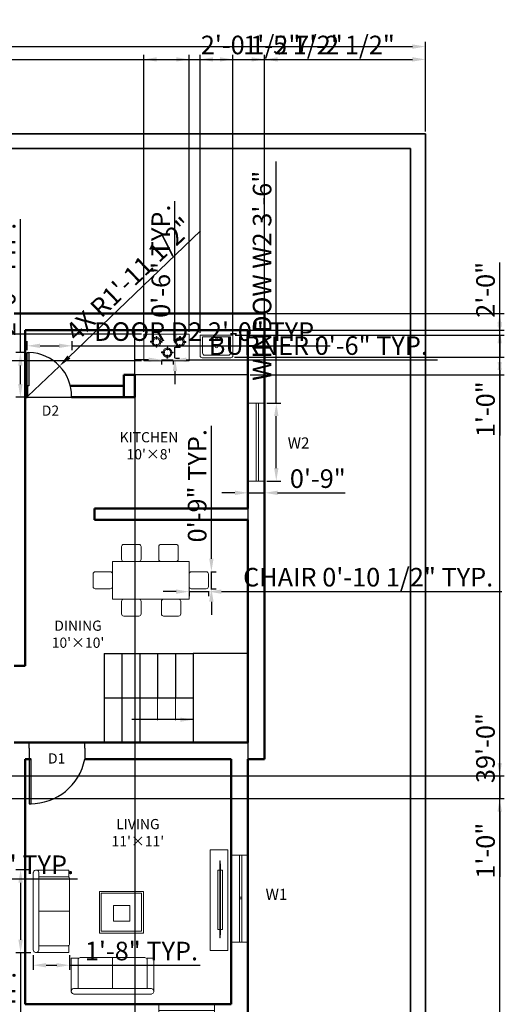
# Model space of a CAD drawing. Units: inches. Extents: x 452 to 1041, y 578 to 1412.
# Tile 3 of 3: x 780 to 1041, y 881 to 1412. Entities that reach past the tile are written whole.
import ezdxf

# ---------------------------------------------------------------- set-up
doc = ezdxf.new("R2010")
doc.units = ezdxf.units.IN
doc.linetypes.add('ACAD_ISO03W100', pattern=[30, 12, -18])
doc.layers.get('Defpoints').update_dxf_attribs({"linetype": 'ACAD_ISO03W100'})
for name, color, linetype, lineweight in [('A-ANNO-DIMS', 2, 'Continuous', 18), ('A-ANNO-SYMB', 7, 'Continuous', 18), ('A-ANNO-TEXT', 7, 'Continuous', 18), ('A-AREA-IDEN', 7, 'Continuous', 25), ('A-DOOR', 3, 'Continuous', 25), ('A-EQPM', 8, 'Continuous', 18), ('A-FLOR-CASE', 8, 'Continuous', 25), ('A-FLOR-FIXT', 9, 'Continuous', 18), ('A-FLOR-STRS', 7, 'Continuous', 25), ('A-FLOR-STRS-OVHD', 7, 'ACAD_ISO03W100', 18), ('A-FURN', 8, 'Continuous', 18), ('A-GLAZ', 160, 'Continuous', 20), ('A-WALL', 7, 'Continuous', 50), ('C-PROP', 7, 'Continuous', 35)]:
    doc.layers.add(name, color=color, linetype=linetype, lineweight=lineweight)
doc.styles.get("Standard").update_dxf_attribs({"font": 'times.ttf'})
doc.dimstyles.new('ISO-25', dxfattribs={"dimscale": 2, "dimtxt": 5, "dimasz": 3.5, "dimexe": 1.25, "dimexo": 0.625, "dimtad": 1, "dimdsep": 46, "dimlunit": 3, "dimtxsty": 'Standard', "dimcen": 2.5, "dimadec": 0, "dimazin": 0, "dimtfac": 1, "dimtmove": 0, "dimatfit": 3, "dimfxl": 1, "dimarcsym": 0})

# ---------------------------------------------------------------- blocks, each defined once
blk = doc.blocks.new('D1')
for p, q in [((734.6, 1191.77), (733.6, 1191.77)), ((733.6, 1191.77), (733.6, 1167.77)), ((734.6, 1161.77), (734.6, 1191.77)), ((704.6, 1161.77), (704.6, 1167.77))]:
    blk.add_line(p, q)
blk.add_arc((733.85, 1161.94), 29.82, 89.5197, 168.7411)
blk = doc.blocks.new('W2')
for p, q in [((902.59, 1205.21), (911.59, 1205.21)), ((907.09, 1163.21), (907.09, 1205.21)), ((908.29, 1163.21), (908.29, 1205.21)), ((911.59, 1205.21), (911.59, 1163.21)), ((902.59, 1163.21), (902.59, 1199.21)), ((911.59, 1163.21), (902.59, 1163.21))]:
    blk.add_line(p, q)
blk = doc.blocks.new('V')
for p, q in [((599.59, 961.66), (599.59, 991.66)), ((599.59, 991.66), (608.59, 991.66)), ((604.09, 961.66), (604.09, 991.66)), ((604.09, 991.66), (605.29, 991.66)), ((605.29, 991.66), (605.29, 961.66)), ((608.59, 991.66), (608.59, 961.66)), ((608.59, 961.66), (599.59, 961.66)), ((608.59, 961.66), (604.09, 961.66))]:
    blk.add_line(p, q)
blk = doc.blocks.new('*D7')
at = {"layer": 'A-ANNO-DIMS', "color": 0, "lineweight": -2, "transparency": 16777216}
for p, q in [((518.29, 1383.36), (518.29, 1399.73)), ((525.29, 1397.23), (991.29, 1397.23)), ((998.29, 1383.36), (998.29, 1399.73))]:
    blk.add_line(p, q, dxfattribs=at)
at = {"layer": 'A-ANNO-DIMS', "color": 0, "lineweight": 70, "transparency": 16777216}
for points in [[(525.29, 1398.4), (525.29, 1396.06), (518.29, 1397.23)], [(991.29, 1398.4), (991.29, 1396.06), (998.29, 1397.23)]]:
    blk.add_solid(points, dxfattribs=at)
at = {"layer": 'Defpoints', "color": 0, "lineweight": 70, "transparency": 16777216}
for p in [(998.29, 1397.23), (518.29, 1382.11), (998.29, 1382.11)]:
    blk.add_point(p, dxfattribs=at)
at = {"layer": 'A-ANNO-DIMS', "color": 0, "transparency": 16777216, "insert": (758.29, 1403.57), "char_height": 10, "attachment_point": 5}
blk.add_mtext("40'", dxfattribs=at)
blk = doc.blocks.new('SOFA-TWO-SEAT')
for p, q in [((0.02, 1.27), (0.02, 19.27)), ((0.02, 19.27), (3.67, 19.27)), ((3.67, 19.27), (3.67, 2.99)), ((3.67, 18.43), (3.67, 17.18)), ((22.25, 19.63), (4.87, 19.63)), ((22.25, 2.99), (22.25, 19.63)), ((22.25, 19.63), (39.61, 19.63)), ((40.81, 2.99), (40.81, 19.27)), ((40.81, 19.27), (44.47, 19.27)), ((40.81, 18.43), (40.81, 15.49)), ((44.47, 19.27), (44.47, 1.51)), ((43.23, 2.99), (1.26, 2.99)), ((1.26, 0.02), (43.23, 0.02))]:
    blk.add_line(p, q)
for centre, radius, start, end in [((4.87, 18.43), 1.2, 90, 180), ((39.61, 18.43), 1.2, 0, 90), ((1.5, 1.51), 1.5, 99.1469, 279.1469), ((42.96, 1.51), 1.51, 259.6305, 79.6305)]:
    blk.add_arc(centre, radius, start, end)
blk = doc.blocks.new('DOOR-D2-24IN')
for p, q in [((0, 0), (0, 24)), ((0, 24), (1, 24)), ((1, 24), (1, 6)), ((1, 6), (0, 6)), ((0, 0), (24, 0))]:
    blk.add_line(p, q)
blk.add_arc((0.44, 0.44), 23.57, 358.9406, 88.6428)
blk = doc.blocks.new('HOB-BURNER')
for points in [[(2.96, 5.87), (3.4, 5.87), (3.4, 4.33), (2.96, 4.33)], [(0, 2.82), (0, 3.26), (1.54, 3.26), (1.54, 2.82)], [(2.89, 1.54), (3.33, 1.54), (3.33, 0), (2.89, 0)], [(4.71, 2.72), (4.71, 3.16), (6.25, 3.16), (6.25, 2.72)]]:
    blk.add_lwpolyline(points, close=True)
for radius, start, end in [(2.46, 93.6474, 171.8424), (2.46, 5.7724, 83.3505), (2.46, 182.15, 264.5703), (1.83, 182.8941, 262.6833), (1.83, 94.9116, 168.9903), (1.83, 276.5524, 353.9094), (2.46, 274.8638, 355.4784), (1.83, 7.7797, 81.0341)]:
    blk.add_arc((3.12, 2.91), radius, start, end)
blk = doc.blocks.new('BASIN-FITTINGS')
blk.add_lwpolyline([(0.26, 5.96), (1.05, 5.96), (1.05, 4.28), (0.26, 4.28)], close=True)
blk.add_circle((0.67, 0.67), 0.671)
blk.add_circle((0.67, 0.67), 0.671)
blk = doc.blocks.new('DINING-CHAIR')
blk.add_lwpolyline([(1.2, 0), (9.27, 0, 0.414214), (10.47, 1.2), (10.47, 7.97, 0.414214), (9.27, 9.17), (1.2, 9.17, 0.414214), (0, 7.97), (0, 1.2, 0.414214)], format="xyb", close=True)
blk = doc.blocks.new('*D18')
at = {"layer": 'A-ANNO-DIMS', "color": 0, "lineweight": -2, "transparency": 16777216}
for p, q in [((917.89, 1205.21), (917.89, 1335.39)), ((912.84, 1205.21), (920.39, 1205.21)), ((917.89, 1170.21), (917.89, 1198.21)), ((912.84, 1163.21), (920.39, 1163.21))]:
    blk.add_line(p, q, dxfattribs=at)
at = {"layer": 'A-ANNO-DIMS', "color": 0, "lineweight": 70, "transparency": 16777216}
for points in [[(916.73, 1198.21), (919.06, 1198.21), (917.89, 1205.21)], [(916.73, 1170.21), (919.06, 1170.21), (917.89, 1163.21)]]:
    blk.add_solid(points, dxfattribs=at)
at = {"layer": 'Defpoints', "color": 0, "lineweight": 70, "transparency": 16777216}
for p in [(911.59, 1205.21), (917.89, 1205.21), (911.59, 1163.21)]:
    blk.add_point(p, dxfattribs=at)
at = {"layer": 'A-ANNO-DIMS', "color": 0, "transparency": 16777216, "insert": (911.53, 1273.8), "char_height": 10, "attachment_point": 5, "rotation": 90}
blk.add_mtext('WINDOW W2 3\'-6"', dxfattribs=at)
blk = doc.blocks.new('*D19')
at = {"layer": 'A-ANNO-DIMS', "color": 0, "lineweight": -2, "transparency": 16777216}
for p, q in [((902.59, 1161.96), (902.59, 1154.41)), ((911.59, 1161.96), (911.59, 1154.41)), ((895.59, 1156.91), (888.59, 1156.91)), ((902.59, 1156.91), (911.59, 1156.91)), ((918.59, 1156.91), (954.95, 1156.91))]:
    blk.add_line(p, q, dxfattribs=at)
at = {"layer": 'A-ANNO-DIMS', "color": 0, "lineweight": 70, "transparency": 16777216}
for points in [[(895.59, 1158.08), (895.59, 1155.74), (902.59, 1156.91)], [(918.59, 1158.08), (918.59, 1155.74), (911.59, 1156.91)]]:
    blk.add_solid(points, dxfattribs=at)
at = {"layer": 'Defpoints', "color": 0, "lineweight": 70, "transparency": 16777216}
for p in [(902.59, 1163.21), (911.59, 1163.21), (911.59, 1156.91)]:
    blk.add_point(p, dxfattribs=at)
at = {"layer": 'A-ANNO-DIMS', "color": 0, "transparency": 16777216, "insert": (940.27, 1163.26), "char_height": 10, "attachment_point": 5}
blk.add_mtext('0\'-9"', dxfattribs=at)
blk = doc.blocks.new('*D23')
at = {"layer": 'A-ANNO-DIMS', "color": 0, "lineweight": -2, "transparency": 16777216}
for p, q in [((708.98, 945.7), (708.98, 951.47)), ((738.98, 945.7), (738.98, 951.47)), ((715.98, 948.97), (731.98, 948.97)), ((738.98, 948.97), (810.77, 948.97))]:
    blk.add_line(p, q, dxfattribs=at)
at = {"layer": 'A-ANNO-DIMS', "color": 0, "lineweight": 70, "transparency": 16777216}
for points in [[(715.98, 950.14), (715.98, 947.8), (708.98, 948.97)], [(731.98, 950.14), (731.98, 947.8), (738.98, 948.97)]]:
    blk.add_solid(points, dxfattribs=at)
at = {"layer": 'Defpoints', "color": 0, "lineweight": 70, "transparency": 16777216}
for p in [(708.98, 944.45), (738.98, 948.97), (738.98, 944.45)]:
    blk.add_point(p, dxfattribs=at)
at = {"layer": 'A-ANNO-DIMS', "color": 0, "transparency": 16777216, "insert": (778.38, 955.32), "char_height": 10, "attachment_point": 5}
blk.add_mtext('2\'-6" TYP.', dxfattribs=at)
blk = doc.blocks.new('*D24')
at = {"layer": 'A-ANNO-DIMS', "color": 0, "lineweight": -2, "transparency": 16777216}
for p, q in [((783.59, 1233.7), (783.59, 1238.59)), ((790.59, 1236.09), (800.84, 1236.09)), ((807.84, 1233.7), (807.84, 1238.59)), ((807.84, 1236.09), (946.96, 1236.09))]:
    blk.add_line(p, q, dxfattribs=at)
at = {"layer": 'A-ANNO-DIMS', "color": 0, "lineweight": 70, "transparency": 16777216}
for points in [[(790.59, 1237.25), (790.59, 1234.92), (783.59, 1236.09)], [(800.84, 1237.25), (800.84, 1234.92), (807.84, 1236.09)]]:
    blk.add_solid(points, dxfattribs=at)
at = {"layer": 'Defpoints', "color": 0, "lineweight": 70, "transparency": 16777216}
for p in [(807.84, 1236.09), (783.59, 1232.45), (807.84, 1232.45)]:
    blk.add_point(p, dxfattribs=at)
at = {"layer": 'A-ANNO-DIMS', "color": 0, "transparency": 16777216, "insert": (880.9, 1242.45), "char_height": 10, "attachment_point": 5}
blk.add_mtext('DOOR D2 2\'-0" TYP.', dxfattribs=at)
blk = doc.blocks.new('*D25')
at = {"layer": 'A-ANNO-DIMS', "color": 0, "lineweight": -2, "transparency": 16777216}
for p, q in [((779.96, 1232.45), (779.96, 1304.24)), ((782.34, 1232.45), (777.46, 1232.45)), ((779.96, 1215.45), (779.96, 1225.45)), ((782.34, 1208.45), (777.46, 1208.45))]:
    blk.add_line(p, q, dxfattribs=at)
at = {"layer": 'A-ANNO-DIMS', "color": 0, "lineweight": 70, "transparency": 16777216}
for points in [[(778.79, 1225.45), (781.12, 1225.45), (779.96, 1232.45)], [(778.79, 1215.45), (781.12, 1215.45), (779.96, 1208.45)]]:
    blk.add_solid(points, dxfattribs=at)
at = {"layer": 'Defpoints', "color": 0, "lineweight": 70, "transparency": 16777216}
for p in [(779.96, 1232.45), (783.59, 1232.45), (783.59, 1208.45)]:
    blk.add_point(p, dxfattribs=at)
at = {"layer": 'A-ANNO-DIMS', "color": 0, "transparency": 16777216, "insert": (773.61, 1271.84), "char_height": 10, "attachment_point": 5, "rotation": 90}
blk.add_mtext('2\'-0" TYP.', dxfattribs=at)
blk = doc.blocks.new('*D28')
at = {"layer": 'A-ANNO-DIMS', "color": 0, "lineweight": -2, "transparency": 16777216}
for p, q in [((849.1, 1228.57), (842.1, 1228.57)), ((856.1, 1228.57), (862.35, 1228.57)), ((856.1, 1228.25), (856.1, 1226.07)), ((862.35, 1228.25), (862.35, 1226.07)), ((869.35, 1228.57), (1004.79, 1228.57))]:
    blk.add_line(p, q, dxfattribs=at)
at = {"layer": 'A-ANNO-DIMS', "color": 0, "lineweight": 70, "transparency": 16777216}
for points in [[(849.1, 1229.73), (849.1, 1227.4), (856.1, 1228.57)], [(869.35, 1229.73), (869.35, 1227.4), (862.35, 1228.57)]]:
    blk.add_solid(points, dxfattribs=at)
at = {"layer": 'Defpoints', "color": 0, "lineweight": 70, "transparency": 16777216}
for p in [(856.1, 1229.5), (862.35, 1229.5), (862.35, 1228.57)]:
    blk.add_point(p, dxfattribs=at)
at = {"layer": 'A-ANNO-DIMS', "color": 0, "transparency": 16777216, "insert": (940.57, 1234.93), "char_height": 10, "attachment_point": 5}
blk.add_mtext('BURNER 0\'-6" TYP.', dxfattribs=at)
blk = doc.blocks.new('*D29')
at = {"layer": 'A-ANNO-DIMS', "color": 0, "lineweight": -2, "transparency": 16777216}
for p, q in [((863.28, 1242.37), (863.28, 1313.94)), ((863.28, 1229.5), (863.28, 1235.37)), ((863.6, 1235.37), (865.78, 1235.37)), ((863.6, 1229.5), (865.78, 1229.5)), ((863.28, 1222.5), (863.28, 1215.5))]:
    blk.add_line(p, q, dxfattribs=at)
at = {"layer": 'A-ANNO-DIMS', "color": 0, "lineweight": 70, "transparency": 16777216}
for points in [[(862.12, 1242.37), (864.45, 1242.37), (863.28, 1235.37)], [(862.12, 1222.5), (864.45, 1222.5), (863.28, 1229.5)]]:
    blk.add_solid(points, dxfattribs=at)
at = {"layer": 'Defpoints', "color": 0, "lineweight": 70, "transparency": 16777216}
for p in [(862.35, 1235.37), (863.28, 1235.37), (862.35, 1229.5)]:
    blk.add_point(p, dxfattribs=at)
at = {"layer": 'A-ANNO-DIMS', "color": 0, "transparency": 16777216, "insert": (856.93, 1281.65), "char_height": 10, "attachment_point": 5, "rotation": 90}
blk.add_mtext('0\'-6" TYP.', dxfattribs=at)
blk = doc.blocks.new('*D32')
at = {"layer": 'A-ANNO-DIMS', "color": 0, "lineweight": -2, "transparency": 16777216}
for p, q in [((785.53, 953.88), (777.57, 953.88)), ((780.07, 946.88), (780.07, 916.19)), ((785.53, 909.19), (777.57, 909.19)), ((780.07, 909.19), (780.07, 774.01))]:
    blk.add_line(p, q, dxfattribs=at)
at = {"layer": 'A-ANNO-DIMS', "color": 0, "lineweight": 70, "transparency": 16777216}
for points in [[(778.91, 946.88), (781.24, 946.88), (780.07, 953.88)], [(778.91, 916.19), (781.24, 916.19), (780.07, 909.19)]]:
    blk.add_solid(points, dxfattribs=at)
at = {"layer": 'Defpoints', "color": 0, "lineweight": 70, "transparency": 16777216}
for p in [(786.78, 953.88), (780.07, 909.19), (786.78, 909.19)]:
    blk.add_point(p, dxfattribs=at)
at = {"layer": 'A-ANNO-DIMS', "color": 0, "transparency": 16777216, "insert": (773.59, 838.1), "char_height": 10, "attachment_point": 5, "rotation": 90}
blk.add_mtext('SOFA 3\'-8 1/2" TYP.', dxfattribs=at)
blk = doc.blocks.new('*D33')
at = {"layer": 'A-ANNO-DIMS', "color": 0, "lineweight": -2, "transparency": 16777216}
for p, q in [((786.78, 907.94), (786.78, 899.99)), ((806.53, 907.94), (806.53, 899.99)), ((793.78, 902.49), (799.53, 902.49)), ((806.53, 902.49), (876.9, 902.49))]:
    blk.add_line(p, q, dxfattribs=at)
at = {"layer": 'A-ANNO-DIMS', "color": 0, "lineweight": 70, "transparency": 16777216}
for points in [[(793.78, 903.65), (793.78, 901.32), (786.78, 902.49)], [(799.53, 903.65), (799.53, 901.32), (806.53, 902.49)]]:
    blk.add_solid(points, dxfattribs=at)
at = {"layer": 'Defpoints', "color": 0, "lineweight": 70, "transparency": 16777216}
for p in [(786.78, 909.19), (806.53, 909.19), (806.53, 902.49)]:
    blk.add_point(p, dxfattribs=at)
at = {"layer": 'A-ANNO-DIMS', "color": 0, "transparency": 16777216, "insert": (845.22, 908.84), "char_height": 10, "attachment_point": 5}
blk.add_mtext('1\'-8" TYP.', dxfattribs=at)
blk = doc.blocks.new('*D36')
at = {"layer": 'A-ANNO-DIMS', "color": 0, "lineweight": -2, "transparency": 16777216}
for p, q in [((863.87, 1103.69), (856.87, 1103.69)), ((870.87, 1104.01), (870.87, 1101.19)), ((870.87, 1103.69), (881.34, 1103.69)), ((881.34, 1104.01), (881.34, 1101.19)), ((888.34, 1103.69), (1039.49, 1103.69))]:
    blk.add_line(p, q, dxfattribs=at)
at = {"layer": 'A-ANNO-DIMS', "color": 0, "lineweight": 70, "transparency": 16777216}
for points in [[(863.87, 1104.86), (863.87, 1102.53), (870.87, 1103.69)], [(888.34, 1104.86), (888.34, 1102.53), (881.34, 1103.69)]]:
    blk.add_solid(points, dxfattribs=at)
at = {"layer": 'Defpoints', "color": 0, "lineweight": 70, "transparency": 16777216}
for p in [(870.87, 1105.26), (881.34, 1105.26), (881.34, 1103.69)]:
    blk.add_point(p, dxfattribs=at)
at = {"layer": 'A-ANNO-DIMS', "color": 0, "transparency": 16777216, "insert": (967.41, 1110.18), "char_height": 10, "attachment_point": 5}
blk.add_mtext('CHAIR 0\'-10 1/2" TYP.', dxfattribs=at)
blk = doc.blocks.new('*D37')
at = {"layer": 'A-ANNO-DIMS', "color": 0, "lineweight": -2, "transparency": 16777216}
for p, q in [((882.91, 1121.44), (882.91, 1193.01)), ((882.59, 1114.44), (885.41, 1114.44)), ((882.91, 1105.26), (882.91, 1114.44)), ((882.59, 1105.26), (885.41, 1105.26)), ((882.91, 1098.26), (882.91, 1091.26))]:
    blk.add_line(p, q, dxfattribs=at)
at = {"layer": 'A-ANNO-DIMS', "color": 0, "lineweight": 70, "transparency": 16777216}
for points in [[(881.75, 1121.44), (884.08, 1121.44), (882.91, 1114.44)], [(881.75, 1098.26), (884.08, 1098.26), (882.91, 1105.26)]]:
    blk.add_solid(points, dxfattribs=at)
at = {"layer": 'Defpoints', "color": 0, "lineweight": 70, "transparency": 16777216}
for p in [(881.34, 1114.44), (882.91, 1114.44), (881.34, 1105.26)]:
    blk.add_point(p, dxfattribs=at)
at = {"layer": 'A-ANNO-DIMS', "color": 0, "transparency": 16777216, "insert": (876.56, 1160.72), "char_height": 10, "attachment_point": 5, "rotation": 90}
blk.add_mtext('0\'-9" TYP.', dxfattribs=at)
blk = doc.blocks.new('*D38')
at = {"layer": 'A-ANNO-DIMS', "color": 0, "lineweight": -2, "transparency": 16777216}
for p, q in [((599.59, 1254.7), (599.59, 1392.83)), ((606.59, 1390.33), (904.59, 1390.33)), ((911.59, 1254.7), (911.59, 1392.83))]:
    blk.add_line(p, q, dxfattribs=at)
at = {"layer": 'A-ANNO-DIMS', "color": 0, "lineweight": 70, "transparency": 16777216}
for points in [[(606.59, 1391.5), (606.59, 1389.17), (599.59, 1390.33)], [(904.59, 1391.5), (904.59, 1389.17), (911.59, 1390.33)]]:
    blk.add_solid(points, dxfattribs=at)
at = {"layer": 'Defpoints', "color": 0, "lineweight": 70, "transparency": 16777216}
for p in [(911.59, 1390.33), (599.59, 1253.45), (911.59, 1253.45)]:
    blk.add_point(p, dxfattribs=at)
at = {"layer": 'A-ANNO-DIMS', "color": 0, "transparency": 16777216, "insert": (755.59, 1396.67), "char_height": 10, "attachment_point": 5}
blk.add_mtext('26\'-0"', dxfattribs=at)
blk = doc.blocks.new('*D39')
at = {"layer": 'A-ANNO-DIMS', "color": 0, "lineweight": -2, "transparency": 16777216}
for p, q in [((912.84, 1253.45), (1040.79, 1253.45)), ((1038.29, 792.45), (1038.29, 1246.45)), ((783.84, 785.45), (1040.79, 785.45))]:
    blk.add_line(p, q, dxfattribs=at)
at = {"layer": 'A-ANNO-DIMS', "color": 0, "lineweight": 70, "transparency": 16777216}
for points in [[(1037.13, 1246.45), (1039.46, 1246.45), (1038.29, 1253.45)], [(1037.13, 792.45), (1039.46, 792.45), (1038.29, 785.45)]]:
    blk.add_solid(points, dxfattribs=at)
at = {"layer": 'Defpoints', "color": 0, "lineweight": 70, "transparency": 16777216}
for p in [(911.59, 1253.45), (1038.29, 1253.45), (782.59, 785.45)]:
    blk.add_point(p, dxfattribs=at)
at = {"layer": 'A-ANNO-DIMS', "color": 0, "transparency": 16777216, "insert": (1031.94, 1019.45), "char_height": 10, "attachment_point": 5, "rotation": 90}
blk.add_mtext('39\'-0"', dxfattribs=at)
blk = doc.blocks.new('*D40')
at = {"layer": 'A-ANNO-DIMS', "color": 0, "lineweight": -2, "transparency": 16777216}
for p, q in [((911.59, 1254.7), (911.59, 1392.83)), ((918.59, 1390.33), (991.29, 1390.33)), ((998.29, 1351.58), (998.29, 1392.83))]:
    blk.add_line(p, q, dxfattribs=at)
at = {"layer": 'A-ANNO-DIMS', "color": 0, "lineweight": 70, "transparency": 16777216}
for points in [[(918.59, 1391.5), (918.59, 1389.17), (911.59, 1390.33)], [(991.29, 1391.5), (991.29, 1389.17), (998.29, 1390.33)]]:
    blk.add_solid(points, dxfattribs=at)
at = {"layer": 'Defpoints', "color": 0, "lineweight": 70, "transparency": 16777216}
for p in [(998.29, 1390.33), (998.29, 1350.33), (911.59, 1253.45)]:
    blk.add_point(p, dxfattribs=at)
at = {"layer": 'A-ANNO-DIMS', "color": 0, "transparency": 16777216, "insert": (954.94, 1396.81), "char_height": 10, "attachment_point": 5}
blk.add_mtext('7\'-2 1/2"', dxfattribs=at)
blk = doc.blocks.new('*D48')
at = {"layer": 'A-ANNO-DIMS', "color": 0, "lineweight": -2, "transparency": 16777216}
for p, q in [((841.74, 1219.2), (841.74, 583.73)), ((902.59, 1219.2), (902.59, 583.73)), ((848.74, 586.23), (895.59, 586.23))]:
    blk.add_line(p, q, dxfattribs=at)
at = {"layer": 'A-ANNO-DIMS', "color": 0, "lineweight": 70, "transparency": 16777216}
for points in [[(848.74, 587.4), (848.74, 585.07), (841.74, 586.23)], [(895.59, 587.4), (895.59, 585.07), (902.59, 586.23)]]:
    blk.add_solid(points, dxfattribs=at)
at = {"layer": 'Defpoints', "color": 0, "lineweight": 70, "transparency": 16777216}
for p in [(841.74, 1220.45), (902.59, 1220.45), (902.59, 586.23)]:
    blk.add_point(p, dxfattribs=at)
at = {"layer": 'A-ANNO-DIMS', "color": 0, "transparency": 16777216, "insert": (872.17, 592.57), "char_height": 10, "attachment_point": 5}
blk.add_mtext('5\'-1"', dxfattribs=at)
blk = doc.blocks.new('*D49')
at = {"layer": 'A-ANNO-DIMS', "color": 0, "lineweight": -2, "transparency": 16777216}
for p, q in [((1038.29, 1244.45), (1038.29, 1281.02)), ((903.84, 1244.45), (1040.79, 1244.45)), ((1038.29, 1227.45), (1038.29, 1237.45)), ((903.84, 1220.45), (1040.79, 1220.45))]:
    blk.add_line(p, q, dxfattribs=at)
at = {"layer": 'A-ANNO-DIMS', "color": 0, "lineweight": 70, "transparency": 16777216}
for points in [[(1037.13, 1237.45), (1039.46, 1237.45), (1038.29, 1244.45)], [(1037.13, 1227.45), (1039.46, 1227.45), (1038.29, 1220.45)]]:
    blk.add_solid(points, dxfattribs=at)
at = {"layer": 'Defpoints', "color": 0, "lineweight": 70, "transparency": 16777216}
for p in [(902.59, 1244.45), (1038.29, 1244.45), (902.59, 1220.45)]:
    blk.add_point(p, dxfattribs=at)
at = {"layer": 'A-ANNO-DIMS', "color": 0, "transparency": 16777216, "insert": (1031.96, 1266.24), "char_height": 10, "attachment_point": 5, "rotation": 90}
blk.add_mtext('2\'-0"', dxfattribs=at)
blk = doc.blocks.new('*D50')
at = {"layer": 'A-ANNO-DIMS', "color": 0, "lineweight": -2, "transparency": 16777216}
for p, q in [((846.47, 1243.68), (846.47, 1392.83)), ((853.47, 1390.33), (863.97, 1390.33)), ((870.97, 1243.68), (870.97, 1392.83)), ((870.97, 1390.33), (930.1, 1390.33))]:
    blk.add_line(p, q, dxfattribs=at)
at = {"layer": 'A-ANNO-DIMS', "color": 0, "lineweight": 70, "transparency": 16777216}
for points in [[(853.47, 1391.5), (853.47, 1389.17), (846.47, 1390.33)], [(863.97, 1391.5), (863.97, 1389.17), (870.97, 1390.33)]]:
    blk.add_solid(points, dxfattribs=at)
at = {"layer": 'Defpoints', "color": 0, "lineweight": 70, "transparency": 16777216}
for p in [(870.97, 1390.33), (846.47, 1242.43), (870.97, 1242.43)]:
    blk.add_point(p, dxfattribs=at)
at = {"layer": 'A-ANNO-DIMS', "color": 0, "transparency": 16777216, "insert": (904.04, 1396.81), "char_height": 10, "attachment_point": 5}
blk.add_mtext('2\'-0 1/2"', dxfattribs=at)
blk = doc.blocks.new('*D51')
at = {"layer": 'A-ANNO-DIMS', "color": 0, "lineweight": -2, "transparency": 16777216}
for p, q in [((478.29, 1249.43), (478.29, 1307.15)), ((845.22, 1242.43), (475.79, 1242.43)), ((478.29, 1228), (478.29, 1242.43)), ((845.22, 1228), (475.79, 1228)), ((478.29, 1221), (478.29, 1214))]:
    blk.add_line(p, q, dxfattribs=at)
at = {"layer": 'A-ANNO-DIMS', "color": 0, "lineweight": 70, "transparency": 16777216}
for points in [[(477.13, 1249.43), (479.46, 1249.43), (478.29, 1242.43)], [(477.13, 1221), (479.46, 1221), (478.29, 1228)]]:
    blk.add_solid(points, dxfattribs=at)
at = {"layer": 'Defpoints', "color": 0, "lineweight": 70, "transparency": 16777216}
for p in [(478.29, 1242.43), (846.47, 1242.43), (846.47, 1228)]:
    blk.add_point(p, dxfattribs=at)
at = {"layer": 'A-ANNO-DIMS', "color": 0, "transparency": 16777216, "insert": (471.82, 1281.79), "char_height": 10, "attachment_point": 5, "rotation": 90}
blk.add_mtext('1\'-2 1/2"', dxfattribs=at)
blk = doc.blocks.new('*D52')
at = {"layer": 'A-ANNO-DIMS', "color": 0, "lineweight": -2, "transparency": 16777216}
for p, q in [((876.81, 1243.11), (876.81, 1392.83)), ((883.81, 1390.33), (887.52, 1390.33)), ((894.52, 1243.11), (894.52, 1392.83)), ((894.52, 1390.33), (952.24, 1390.33))]:
    blk.add_line(p, q, dxfattribs=at)
at = {"layer": 'A-ANNO-DIMS', "color": 0, "lineweight": 70, "transparency": 16777216}
for points in [[(883.81, 1391.5), (883.81, 1389.17), (876.81, 1390.33)], [(887.52, 1391.5), (887.52, 1389.17), (894.52, 1390.33)]]:
    blk.add_solid(points, dxfattribs=at)
at = {"layer": 'Defpoints', "color": 0, "lineweight": 70, "transparency": 16777216}
for p in [(894.52, 1390.33), (876.81, 1241.86), (894.52, 1241.86)]:
    blk.add_point(p, dxfattribs=at)
at = {"layer": 'A-ANNO-DIMS', "color": 0, "transparency": 16777216, "insert": (926.88, 1396.81), "char_height": 10, "attachment_point": 5}
blk.add_mtext('1\'-5 1/2"', dxfattribs=at)
blk = doc.blocks.new('*D53')
at = {"layer": 'A-ANNO-DIMS', "color": 0, "lineweight": -2, "transparency": 16777216}
for p, q in [((1038.29, 1248.86), (1038.29, 1255.86)), ((895.77, 1241.86), (1040.79, 1241.86)), ((1038.29, 1241.86), (1038.29, 1230.01)), ((895.42, 1230.01), (1040.79, 1230.01)), ((1038.29, 1223.01), (1038.29, 1187.85))]:
    blk.add_line(p, q, dxfattribs=at)
at = {"layer": 'A-ANNO-DIMS', "color": 0, "lineweight": 70, "transparency": 16777216}
for points in [[(1037.13, 1248.86), (1039.46, 1248.86), (1038.29, 1241.86)], [(1037.13, 1223.01), (1039.46, 1223.01), (1038.29, 1230.01)]]:
    blk.add_solid(points, dxfattribs=at)
at = {"layer": 'Defpoints', "color": 0, "lineweight": 70, "transparency": 16777216}
for p in [(894.52, 1241.86), (894.17, 1230.01), (1038.29, 1230.01)]:
    blk.add_point(p, dxfattribs=at)
at = {"layer": 'A-ANNO-DIMS', "color": 0, "transparency": 16777216, "insert": (1031.96, 1201.93), "char_height": 10, "attachment_point": 5, "rotation": 90}
blk.add_mtext('1\'-0"', dxfattribs=at)
blk = doc.blocks.new('*D57')
at = {"layer": 'A-ANNO-DIMS', "color": 0, "lineweight": -2, "transparency": 16777216}
for p, q in [((1038.29, 1011.45), (1038.29, 1018.45)), ((666.18, 1004.45), (1040.79, 1004.45)), ((1038.29, 1004.45), (1038.29, 992.25)), ((664.98, 992.25), (1040.79, 992.25)), ((1038.29, 985.25), (1038.29, 950.09))]:
    blk.add_line(p, q, dxfattribs=at)
at = {"layer": 'A-ANNO-DIMS', "color": 0, "lineweight": 70, "transparency": 16777216}
for points in [[(1037.13, 1011.45), (1039.46, 1011.45), (1038.29, 1004.45)], [(1037.13, 985.25), (1039.46, 985.25), (1038.29, 992.25)]]:
    blk.add_solid(points, dxfattribs=at)
at = {"layer": 'Defpoints', "color": 0, "lineweight": 70, "transparency": 16777216}
for p in [(664.93, 1004.45), (663.73, 992.25), (1038.29, 992.25)]:
    blk.add_point(p, dxfattribs=at)
at = {"layer": 'A-ANNO-DIMS', "color": 0, "transparency": 16777216, "insert": (1031.96, 964.17), "char_height": 10, "attachment_point": 5, "rotation": 90}
blk.add_mtext('1\'-0"', dxfattribs=at)
blk = doc.blocks.new('*D59')
at = {"layer": 'A-ANNO-DIMS', "color": 0, "lineweight": -2, "transparency": 16777216}
for p, q in [((876.98, 1297.99), (806.1, 1230.04)), ((784.04, 1208.89), (801.05, 1225.2))]:
    blk.add_line(p, q, dxfattribs=at)
at = {"layer": 'A-ANNO-DIMS', "color": 0, "lineweight": 70, "transparency": 16777216}
blk.add_solid([(805.3, 1230.88), (806.91, 1229.2), (801.05, 1225.2)], dxfattribs=at)
at = {"layer": 'Defpoints', "color": 0, "lineweight": 70, "transparency": 16777216}
for p in [(801.05, 1225.2), (784.04, 1208.89)]:
    blk.add_point(p, dxfattribs=at)
at = {"layer": 'A-ANNO-DIMS', "color": 0, "transparency": 16777216, "insert": (839.59, 1271.11), "char_height": 10, "attachment_point": 5, "rotation": 43.7912}
blk.add_mtext('4X R1\'-11 1/2"', dxfattribs=at)

msp = doc.modelspace()

# ---------------------------------------------------------------- linework, layer by layer
at = {"layer": 'A-DOOR'}
for p, q in [((784.712, 1019.451), (784.712, 1022.451)), ((814.712, 1019.451), (814.712, 1022.451))]:
    msp.add_line(p, q, dxfattribs=at)
at = {"layer": 'A-EQPM'}
msp.add_lwpolyline([(870.971, 1242.43), (846.468, 1242.43), (846.468, 1228.003), (870.971, 1228.003)], close=True, dxfattribs=at)
at = {"layer": 'A-FLOR-CASE'}
for p, q in [((841.739, 1220.451), (841.739, 1244.451)), ((902.593, 1244.451), (902.593, 1214.451)), ((902.593, 1244.451), (902.593, 1220.451)), ((902.593, 1220.451), (841.739, 1220.451))]:
    msp.add_line(p, q, dxfattribs=at)
at = {"layer": 'A-FLOR-FIXT'}
for points in [[(876.807, 1241.863), (894.519, 1241.863), (894.519, 1230.863, -0.4142136), (893.319, 1229.663), (878.007, 1229.663, -0.4142136), (876.807, 1230.863)], [(878.177, 1240.907), (893.272, 1240.907), (893.272, 1232.24, -0.4142136), (892.072, 1231.04), (879.377, 1231.04, -0.4142136), (878.177, 1232.24)]]:
    msp.add_lwpolyline(points, format="xyb", close=True, dxfattribs=at)
at = {"layer": 'A-FLOR-STRS'}
for p, q in [((825.093, 1070.451), (825.093, 1022.451)), ((825.093, 1070.451), (873.093, 1070.451)), ((834.693, 1070.451), (834.693, 1022.451)), ((844.293, 1070.451), (844.293, 1022.451)), ((853.893, 1070.451), (853.893, 1046.451)), ((863.493, 1070.451), (863.493, 1046.451)), ((902.593, 1070.451), (873.093, 1070.451)), ((873.093, 1070.451), (873.093, 1022.451)), ((902.593, 1022.451), (902.593, 1070.451)), ((825.093, 1046.451), (873.093, 1046.451))]:
    msp.add_line(p, q, dxfattribs=at)
at = {"layer": 'A-FLOR-STRS-OVHD'}
for p, q in [((853.893, 1046.451), (853.893, 1022.451)), ((863.493, 1046.451), (863.493, 1022.451))]:
    msp.add_line(p, q, dxfattribs=at)
at = {"layer": 'A-FURN'}
for p, q in [((887.459, 958.775), (887.459, 917.276)), ((887.459, 958.775), (887.715, 958.775)), ((887.715, 958.775), (887.715, 917.276)), ((887.715, 957.095), (887.715, 957.081)), ((887.715, 957.081), (887.899, 957.081)), ((887.899, 957.081), (887.899, 918.793)), ((887.459, 953.618), (886.427, 953.618)), ((886.427, 953.618), (886.427, 921.719)), ((887.899, 953.647), (888.836, 953.647)), ((888.836, 953.647), (888.836, 921.748)), ((886.427, 921.719), (887.459, 921.719)), ((887.899, 918.793), (887.715, 918.793)), ((888.836, 921.748), (887.899, 921.748)), ((887.715, 917.276), (887.459, 917.276))]:
    msp.add_line(p, q, dxfattribs=at)
for points in [[(855.78, 1119.995), (863.853, 1119.995, 0.4142136), (865.053, 1121.195), (865.053, 1127.97, 0.4142136), (863.853, 1129.17), (855.78, 1129.17, 0.4142136), (854.58, 1127.97), (854.58, 1121.195, 0.4142136)], [(820.348, 1105.265), (828.422, 1105.265, 0.4142136), (829.622, 1106.465), (829.622, 1113.239, 0.4142136), (828.422, 1114.439), (820.348, 1114.439, 0.4142136), (819.148, 1113.239), (819.148, 1106.465, 0.4142136)], [(835.735, 1090.534), (843.809, 1090.534, 0.4142136), (845.009, 1091.734), (845.009, 1098.508, 0.4142136), (843.809, 1099.708), (835.735, 1099.708, 0.4142136), (834.535, 1098.508), (834.535, 1091.734, 0.4142136)], [(857.157, 1090.534), (865.23, 1090.534, 0.4142136), (866.43, 1091.734), (866.43, 1098.508, 0.4142136), (865.23, 1099.708), (857.157, 1099.708, 0.4142136), (855.957, 1098.508), (855.957, 1091.734, 0.4142136)]]:
    msp.add_lwpolyline(points, format="xyb", close=True, dxfattribs=at)
for points in [[(829.622, 1119.995), (870.869, 1119.995), (870.869, 1099.708), (829.622, 1099.708)], [(882.334, 964.561), (891.865, 964.561), (891.865, 910.453), (882.334, 910.453)], [(822.56, 942.175), (846.349, 942.175), (846.349, 919.812), (822.56, 919.812)], [(823.466, 941.265), (845.249, 941.265), (845.249, 920.779), (823.466, 920.779)], [(830.221, 934.698), (838.921, 934.698), (838.921, 926.161), (830.221, 926.161)]]:
    msp.add_lwpolyline(points, close=True, dxfattribs=at)
at = {"layer": 'A-GLAZ'}
for p, q in [((902.593, 1199.211), (902.593, 1205.211)), ((893.593, 914.932), (893.593, 961.732)), ((893.593, 961.732), (902.593, 961.732)), ((898.093, 961.732), (898.093, 914.932)), ((899.293, 961.732), (899.293, 914.932)), ((902.593, 961.732), (902.593, 914.932)), ((898.093, 939.13), (899.293, 939.13)), ((898.093, 938.332), (899.293, 938.332)), ((902.593, 914.932), (893.593, 914.932))]:
    msp.add_line(p, q, dxfattribs=at)
at = {"layer": 'A-WALL'}
for p, q in [((776.593, 1253.451), (782.593, 1253.451)), ((782.593, 1253.451), (902.593, 1253.451)), ((902.593, 1253.451), (911.593, 1253.451)), ((911.593, 1253.451), (911.593, 1148.451)), ((782.593, 1244.451), (782.593, 1142.451)), ((782.593, 1244.451), (902.593, 1244.451)), ((902.593, 1244.451), (902.593, 1148.451)), ((841.739, 1220.451), (835.739, 1220.451)), ((835.739, 1220.451), (835.739, 1208.451)), ((841.739, 1220.451), (841.739, 1208.451)), ((783.593, 1214.451), (782.593, 1214.451)), ((783.593, 1208.451), (783.593, 1214.451)), ((806.94, 1214.451), (835.739, 1214.451)), ((782.593, 1208.451), (783.593, 1208.451)), ((835.739, 1208.451), (807.593, 1208.451)), ((835.739, 1208.451), (841.739, 1208.451)), ((902.593, 1148.451), (819.893, 1148.451)), ((819.893, 1148.451), (819.893, 1142.451)), ((911.593, 1148.451), (911.593, 1142.451)), ((782.593, 1063.736), (782.593, 1142.451)), ((902.593, 1142.451), (819.893, 1142.451)), ((902.593, 1142.451), (902.593, 1022.451)), ((911.593, 1142.451), (911.593, 1022.451)), ((776.593, 1063.736), (782.593, 1063.736)), ((902.593, 1022.451), (776.593, 1022.451)), ((911.593, 1022.451), (911.593, 1013.451)), ((782.593, 881.451), (782.593, 1013.451)), ((785.712, 1013.451), (782.593, 1013.451)), ((893.593, 1013.451), (814.712, 1013.451)), ((893.593, 1013.451), (893.593, 881.451)), ((911.593, 1013.451), (902.593, 1013.451)), ((902.593, 1013.451), (902.593, 872.451)), ((893.593, 881.451), (782.593, 881.451)), ((893.593, 881.451), (782.593, 881.451))]:
    msp.add_line(p, q, dxfattribs=at)
at = {"layer": 'C-PROP'}
for p, q in [((518.294, 1350.334), (998.294, 1350.334)), ((998.294, 1350.334), (998.294, 630.334)), ((526.294, 1342.334), (990.294, 1342.334)), ((990.294, 1342.334), (990.294, 638.334))]:
    msp.add_line(p, q, dxfattribs=at)

# ---------------------------------------------------------------- block references
at = {"layer": 'A-DOOR'}
msp.add_blockref('DOOR-D2-24IN', (783.593, 1208.451), dxfattribs=at)
at = {"layer": 'A-DOOR', "rotation": 180}
msp.add_blockref('D1', (1519.31, 2181.218), dxfattribs=at)
at = {"layer": 'A-EQPM'}
for p in [(850.182, 1235.316), (862.822, 1235.186), (856.096, 1229.504)]:
    msp.add_blockref('HOB-BURNER', p, dxfattribs=at)
at = {"layer": 'A-FLOR-FIXT'}
msp.add_blockref('BASIN-FITTINGS', (885.005, 1234.942), dxfattribs=at)
at = {"layer": 'A-FURN'}
for name, p in [('DINING-CHAIR', (834.535, 1119.995)), ('DINING-CHAIR', (870.869, 1105.264)), ('SOFA-TWO-SEAT', (807.405, 886.971))]:
    msp.add_blockref(name, p, dxfattribs=at)
at = {"layer": 'A-FURN', "rotation": 269.999999999999}
msp.add_blockref('SOFA-TWO-SEAT', (786.902, 953.786), dxfattribs=at)
at = {"layer": 'A-GLAZ'}
msp.add_blockref('W2', (0, 0), dxfattribs=at)
at = {"layer": 'A-GLAZ', "rotation": 90}
msp.add_blockref('V', (1846.252, 272.857), dxfattribs=at)

# ---------------------------------------------------------------- texts
at = {"layer": 'A-ANNO-TEXT', "attachment_point": 1}
for s, insert, char_height in [('D2', (791.52, 1203.92), 5.5), ('W2', (924.056, 1186.758), 6), ('D1', (794.88, 1016.625), 5.5), ('W1', (912.131, 943.648), 6)]:
    msp.add_mtext_dynamic_manual_height_columns(s, width=337.44086, gutter_width=12.5, heights=[0], dxfattribs=dict(at, insert=insert, char_height=char_height))
at = {"layer": 'A-AREA-IDEN', "char_height": 5.5, "attachment_point": 1}
for s, insert in [("\\pxqc;KITCHEN\\P10'×8'", (680.556, 1189.604)), ("\\pxqc;DINING\\P10'×10'", (642.321, 1088.11)), ("\\pxqc;LIVING \\P11'×11'", (674.581, 981.244))]:
    msp.add_mtext_dynamic_manual_height_columns(s, width=337.44086, gutter_width=12.5, heights=[0], dxfattribs=dict(at, insert=insert))

# ---------------------------------------------------------------- dimensions: what is measured, and where the dimension line sits
at = {"layer": 'A-ANNO-DIMS'}
for base, p1, p2, override, picture, middle in [((870.971, 1390.334), (846.468, 1242.43), (870.971, 1242.43), {"dimdec": 1, "dimlfac": 1, "dimrnd": 0, "dimzin": 1, "dimdsep": 46, "dimlunit": 4, "dimfrac": 2}, '*D50', (904.037, 1396.811)), ((894.519, 1390.334), (876.807, 1241.863), (894.519, 1241.863), {"dimdec": 1, "dimlfac": 1, "dimrnd": 0, "dimzin": 1, "dimdsep": 46, "dimlunit": 4, "dimfrac": 2}, '*D52', (926.879, 1396.811)), ((998.294, 1390.334), (911.593, 1253.451), (998.294, 1350.334), {"dimdec": 1, "dimlfac": 1, "dimrnd": 0, "dimzin": 1, "dimdsep": 46, "dimlunit": 4, "dimfrac": 2}, '*D40', (954.944, 1396.811)), ((998.294, 1397.23), (518.294, 1382.109), (998.294, 1382.109), {"dimclrd": 0, "dimclre": 0, "dimclrt": 0}, '*D7', (758.294, 1403.567)), ((911.593, 1390.334), (599.593, 1253.451), (911.593, 1253.451), {"dimdec": 1, "dimlfac": 1, "dimrnd": 0, "dimzin": 1, "dimdsep": 46, "dimlunit": 4, "dimfrac": 2}, '*D38', (755.593, 1396.671)), ((902.593, 586.234), (841.739, 1220.451), (902.593, 1220.451), {"dimdec": 1, "dimlfac": 1, "dimrnd": 0, "dimzin": 1, "dimdsep": 46, "dimlunit": 4, "dimfrac": 2}, '*D48', (872.166, 592.571)), ((911.593, 1156.911), (902.593, 1163.211), (911.593, 1163.211), {"dimdec": 1, "dimlfac": 1, "dimrnd": 0, "dimzin": 1, "dimdsep": 46, "dimlunit": 4, "dimfrac": 2}, '*D19', (940.272, 1163.262))]:
    dim = msp.add_linear_dim(base=base, p1=p1, p2=p2, dimstyle='ISO-25', override=override, dxfattribs=at)
    dim.commit()
    dim.dimension.update_dxf_attribs({"geometry": picture, "text_midpoint": middle})
for base, p1, p2, angle, text, picture, middle in [((917.893, 1205.211), (911.593, 1163.211), (911.593, 1205.211), 90, 'WINDOW W2 <>', '*D18', (911.532, 1273.8)), ((863.283, 1235.369), (862.345, 1229.504), (862.345, 1235.369), 90, '<> TYP.', '*D29', (856.932, 1281.654)), ((779.956, 1232.451), (783.593, 1208.451), (783.593, 1232.451), 90, '<> TYP.', '*D25', (773.605, 1271.843)), ((882.913, 1114.439), (881.342, 1105.265), (881.342, 1114.439), 90, '<> TYP.', '*D37', (876.562, 1160.724)), ((780.074, 909.191), (786.777, 953.88), (786.777, 909.191), 270, 'SOFA <> TYP.', '*D32', (773.586, 838.101))]:
    dim = msp.add_linear_dim(base=base, p1=p1, p2=p2, angle=angle, text=text, dimstyle='ISO-25', override={"dimdec": 1, "dimlfac": 1, "dimrnd": 0, "dimzin": 1, "dimdsep": 46, "dimlunit": 4, "dimfrac": 2}, dxfattribs=at)
    dim.commit()
    dim.dimension.update_dxf_attribs({"geometry": picture, "text_midpoint": middle})
for base, p1, p2, picture, middle in [((478.294, 1242.43), (846.468, 1228.003), (846.468, 1242.43), '*D51', (471.817, 1281.79)), ((1038.294, 1244.451), (902.593, 1220.451), (902.593, 1244.451), '*D49', (1031.958, 1266.237)), ((1038.294, 1253.451), (782.593, 785.451), (911.593, 1253.451), '*D39', (1031.943, 1019.451)), ((1038.294, 1230.014), (894.519, 1241.863), (894.168, 1230.014), '*D53', (1031.958, 1201.934)), ((1038.294, 992.251), (664.929, 1004.451), (663.729, 992.251), '*D57', (1031.958, 964.171))]:
    dim = msp.add_linear_dim(base=base, p1=p1, p2=p2, angle=90, dimstyle='ISO-25', override={"dimdec": 1, "dimlfac": 1, "dimrnd": 0, "dimzin": 1, "dimdsep": 46, "dimlunit": 4, "dimfrac": 2}, dxfattribs=at)
    dim.commit()
    dim.dimension.update_dxf_attribs({"geometry": picture, "text_midpoint": middle})
dim = msp.add_radius_dim(center=(784.035, 1208.886), mpoint=(801.05, 1225.198), text='4X <>', dimstyle='ISO-25', override={"dimdec": 1, "dimlfac": 1, "dimrnd": 0, "dimzin": 1, "dimdsep": 46, "dimlunit": 4, "dimfrac": 2}, dxfattribs=at)
dim.commit()
dim.dimension.update_dxf_attribs({"geometry": '*D59', "text_midpoint": (839.587, 1271.115)})
for base, p1, p2, text, picture, middle in [((807.842, 1236.088), (783.593, 1232.451), (807.842, 1232.451), 'DOOR D2 <> TYP.', '*D24', (880.901, 1242.45)), ((862.345, 1228.566), (856.096, 1229.504), (862.345, 1229.504), 'BURNER <> TYP.', '*D28', (940.566, 1234.932)), ((881.342, 1103.694), (870.869, 1105.265), (881.342, 1105.265), 'CHAIR <> TYP.', '*D36', (967.414, 1110.182)), ((738.984, 948.969), (708.984, 944.451), (738.984, 944.451), '<> TYP.', '*D23', (778.376, 955.32)), ((806.532, 902.488), (786.777, 909.191), (806.532, 909.191), '<> TYP.', '*D33', (845.218, 908.839))]:
    dim = msp.add_linear_dim(base=base, p1=p1, p2=p2, text=text, dimstyle='ISO-25', override={"dimdec": 1, "dimlfac": 1, "dimrnd": 0, "dimzin": 1, "dimdsep": 46, "dimlunit": 4, "dimfrac": 2}, dxfattribs=at)
    dim.commit()
    dim.dimension.update_dxf_attribs({"geometry": picture, "text_midpoint": middle})

# ---------------------------------------------------------------- leaders
at = {"layer": 'A-ANNO-SYMB'}
msp.add_leader([(873.093, 1034.755), (839.963, 1034.755)], dimstyle='ISO-25', dxfattribs=at)

doc.saveas('drawing.dxf')
